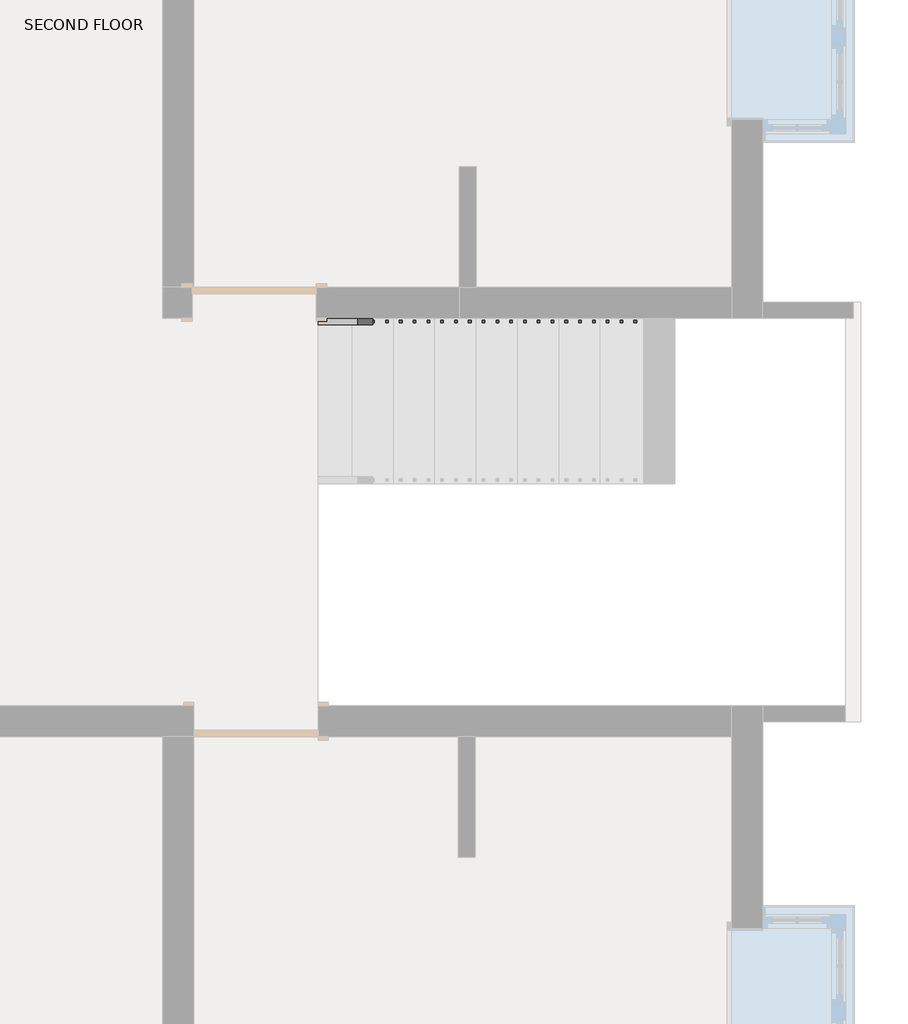
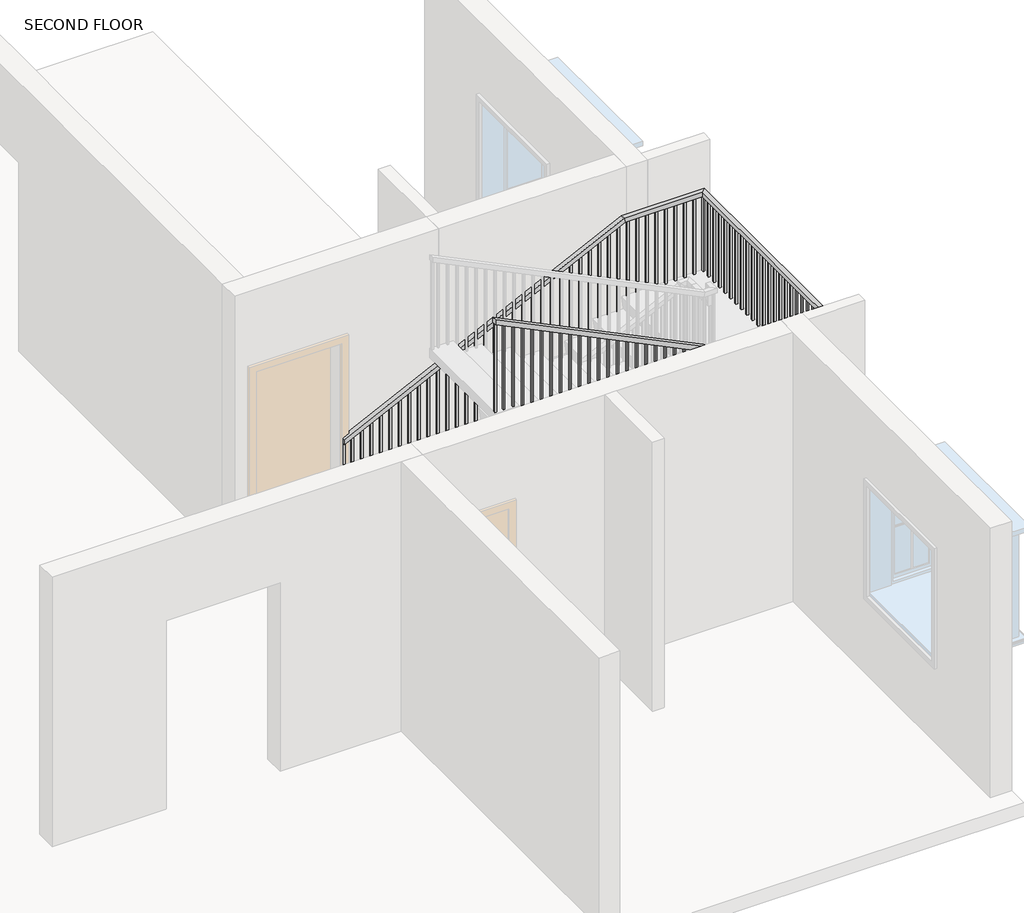
# One storey, part 4 of 6: 1 railing.
"""IFC4 building model written with IfcOpenShell, lengths in millimetres."""

from ifc_helpers import new_model, si_unit, frame, origin, place, context, project, spatial, polyline, outline, extrude, faceted_brep, element, save

model = new_model("IFC4")

# Units and contexts
model_context = context("Model", 3, world=origin())
ifc_project = project(units=[si_unit("LENGTHUNIT", "METRE", prefix="MILLI")], contexts=[model_context])

# Site, building, storey
site = spatial("IfcSite", under=ifc_project)
building = spatial("IfcBuilding", under=site)
storey = spatial("IfcBuildingStorey", under=building, Name="SECOND FLOOR", Elevation=6400.8)

# Railing
placement = place(None, origin())
element("IfcRailing", 1, ObjectType="Handrail - Rectangular", at=placement, inside=storey, context=model_context, shape_type="SolidModel", body=[
    faceted_brep([(3126.2584916, 220.733346, 7460.6727273), (3126.2584916, 220.733346, 7404.1956113), (3126.2584916, 169.933346, 7404.1956113), (3126.2584916, 169.933346, 7460.6727273), (6120.7829507, 220.733346, 8915.4), (6132.4691705, 220.733346, 8864.6), (6132.4691705, 169.933346, 8864.6), (6120.7829507, 169.933346, 8915.4), (7009.1350459, 220.733346, 8915.4), (7009.1350459, 220.733346, 8864.6), (6958.3350459, 169.933346, 8864.6), (6958.3350459, 169.933346, 8915.4), (7009.1350459, -2636.766654, 8915.4), (7009.1350459, -2636.766654, 8864.6), (6958.3350459, -2585.966654, 8864.6), (6958.3350459, -2585.966654, 8915.4), (6420.2353966, -2636.766654, 8915.4), (6408.5491768, -2636.766654, 8864.6), (6408.5491768, -2585.966654, 8864.6), (6420.2353966, -2585.966654, 8915.4), (3126.2584916, -2636.766654, 10515.6), (3126.2584916, -2585.966654, 10515.6), (3126.2584916, -2585.966654, 10459.122884), (3126.2584916, -2636.766654, 10459.122884)], [[[0, 1, 2, 3]], [[1, 0, 4, 5]], [[2, 1, 5, 6]], [[3, 2, 6, 7]], [[0, 3, 7, 4]], [[5, 4, 8, 9]], [[6, 5, 9, 10]], [[7, 6, 10, 11]], [[4, 7, 11, 8]], [[9, 8, 12, 13]], [[10, 9, 13, 14]], [[11, 10, 14, 15]], [[8, 11, 15, 12]], [[13, 12, 16, 17]], [[14, 13, 17, 18]], [[15, 14, 18, 19]], [[12, 15, 19, 16]], [[20, 21, 22, 23]], [[17, 16, 20, 23]], [[18, 17, 23, 22]], [[19, 18, 22, 21]], [[16, 19, 21, 20]]]),
    extrude(outline(polyline([(10416.0077556, 3215.0100459), (9455.7272727, 3215.0100459), (9455.7272727, 3234.0600459), (10406.7533465, 3234.0600459), (10416.0077556, 3215.0100459)])), frame((0.0, -2620.891654, 0.0), z_axis=(0.0, 1.0, 0.0), x_axis=(0.0, 0.0, 1.0)), (0.0, 0.0, 1.0), 19.05),
    extrude(outline(polyline([(10366.6509068, 3316.6100459), (9455.7272727, 3316.6100459), (9455.7272727, 3335.6600459), (10357.3964977, 3335.6600459), (10366.6509068, 3316.6100459)])), frame((0.0, -2620.891654, 0.0), z_axis=(0.0, 1.0, 0.0), x_axis=(0.0, 0.0, 1.0)), (0.0, 0.0, 1.0), 19.05),
    extrude(outline(polyline([(10317.294058, 3418.2100459), (9310.2545455, 3418.2100459), (9310.2545455, 3437.2600459), (10308.0396489, 3437.2600459), (10317.294058, 3418.2100459)])), frame((0.0, -2620.891654, 0.0), z_axis=(0.0, 1.0, 0.0), x_axis=(0.0, 0.0, 1.0)), (0.0, 0.0, 1.0), 19.05),
    extrude(outline(polyline([(10267.9372093, 3519.8100459), (9310.2545455, 3519.8100459), (9310.2545455, 3538.8600459), (10258.6828001, 3538.8600459), (10267.9372093, 3519.8100459)])), frame((0.0, -2620.891654, 0.0), z_axis=(0.0, 1.0, 0.0), x_axis=(0.0, 0.0, 1.0)), (0.0, 0.0, 1.0), 19.05),
    extrude(outline(polyline([(10218.5803605, 3621.4100459), (9310.2545455, 3621.4100459), (9310.2545455, 3640.4600459), (10209.3259513, 3640.4600459), (10218.5803605, 3621.4100459)])), frame((0.0, -2620.891654, 0.0), z_axis=(0.0, 1.0, 0.0), x_axis=(0.0, 0.0, 1.0)), (0.0, 0.0, 1.0), 19.05),
    extrude(outline(polyline([(10169.2235117, 3723.0100459), (9164.7818182, 3723.0100459), (9164.7818182, 3742.0600459), (10159.9691025, 3742.0600459), (10169.2235117, 3723.0100459)])), frame((0.0, -2620.891654, 0.0), z_axis=(0.0, 1.0, 0.0), x_axis=(0.0, 0.0, 1.0)), (0.0, 0.0, 1.0), 19.05),
    extrude(outline(polyline([(10119.8666629, 3824.6100459), (9164.7818182, 3824.6100459), (9164.7818182, 3843.6600459), (10110.6122538, 3843.6600459), (10119.8666629, 3824.6100459)])), frame((0.0, -2620.891654, 0.0), z_axis=(0.0, 1.0, 0.0), x_axis=(0.0, 0.0, 1.0)), (0.0, 0.0, 1.0), 19.05),
    extrude(outline(polyline([(10070.5098141, 3926.2100459), (9164.7818182, 3926.2100459), (9164.7818182, 3945.2600459), (10061.255405, 3945.2600459), (10070.5098141, 3926.2100459)])), frame((0.0, -2620.891654, 0.0), z_axis=(0.0, 1.0, 0.0), x_axis=(0.0, 0.0, 1.0)), (0.0, 0.0, 1.0), 19.05),
    extrude(outline(polyline([(10021.1529653, 4027.8100459), (9019.3090909, 4027.8100459), (9019.3090909, 4046.8600459), (10011.8985562, 4046.8600459), (10021.1529653, 4027.8100459)])), frame((0.0, -2620.891654, 0.0), z_axis=(0.0, 1.0, 0.0), x_axis=(0.0, 0.0, 1.0)), (0.0, 0.0, 1.0), 19.05),
    extrude(outline(polyline([(9971.7961165, 4129.4100459), (9019.3090909, 4129.4100459), (9019.3090909, 4148.4600459), (9962.5417074, 4148.4600459), (9971.7961165, 4129.4100459)])), frame((0.0, -2620.891654, 0.0), z_axis=(0.0, 1.0, 0.0), x_axis=(0.0, 0.0, 1.0)), (0.0, 0.0, 1.0), 19.05),
    extrude(outline(polyline([(9922.4392678, 4231.0100459), (9019.3090909, 4231.0100459), (9019.3090909, 4250.0600459), (9913.1848586, 4250.0600459), (9922.4392678, 4231.0100459)])), frame((0.0, -2620.891654, 0.0), z_axis=(0.0, 1.0, 0.0), x_axis=(0.0, 0.0, 1.0)), (0.0, 0.0, 1.0), 19.05),
    extrude(outline(polyline([(9873.082419, 4332.6100459), (8873.8363636, 4332.6100459), (8873.8363636, 4351.6600459), (9863.8280098, 4351.6600459), (9873.082419, 4332.6100459)])), frame((0.0, -2620.891654, 0.0), z_axis=(0.0, 1.0, 0.0), x_axis=(0.0, 0.0, 1.0)), (0.0, 0.0, 1.0), 19.05),
    extrude(outline(polyline([(9823.7255702, 4434.2100459), (8873.8363636, 4434.2100459), (8873.8363636, 4453.2600459), (9814.471161, 4453.2600459), (9823.7255702, 4434.2100459)])), frame((0.0, -2620.891654, 0.0), z_axis=(0.0, 1.0, 0.0), x_axis=(0.0, 0.0, 1.0)), (0.0, 0.0, 1.0), 19.05),
    extrude(outline(polyline([(9774.3687214, 4535.8100459), (8873.8363636, 4535.8100459), (8873.8363636, 4554.8600459), (9765.1143123, 4554.8600459), (9774.3687214, 4535.8100459)])), frame((0.0, -2620.891654, 0.0), z_axis=(0.0, 1.0, 0.0), x_axis=(0.0, 0.0, 1.0)), (0.0, 0.0, 1.0), 19.05),
    extrude(outline(polyline([(9725.0118726, 4637.4100459), (8728.3636364, 4637.4100459), (8728.3636364, 4656.4600459), (9715.7574635, 4656.4600459), (9725.0118726, 4637.4100459)])), frame((0.0, -2620.891654, 0.0), z_axis=(0.0, 1.0, 0.0), x_axis=(0.0, 0.0, 1.0)), (0.0, 0.0, 1.0), 19.05),
    extrude(outline(polyline([(9675.6550238, 4739.0100459), (8728.3636364, 4739.0100459), (8728.3636364, 4758.0600459), (9666.4006147, 4758.0600459), (9675.6550238, 4739.0100459)])), frame((0.0, -2620.891654, 0.0), z_axis=(0.0, 1.0, 0.0), x_axis=(0.0, 0.0, 1.0)), (0.0, 0.0, 1.0), 19.05),
    extrude(outline(polyline([(9626.2981751, 4840.6100459), (8728.3636364, 4840.6100459), (8728.3636364, 4859.6600459), (9617.0437659, 4859.6600459), (9626.2981751, 4840.6100459)])), frame((0.0, -2620.891654, 0.0), z_axis=(0.0, 1.0, 0.0), x_axis=(0.0, 0.0, 1.0)), (0.0, 0.0, 1.0), 19.05),
    extrude(outline(polyline([(9576.9413263, 4942.2100459), (8582.8909091, 4942.2100459), (8582.8909091, 4961.2600459), (9567.6869171, 4961.2600459), (9576.9413263, 4942.2100459)])), frame((0.0, -2620.891654, 0.0), z_axis=(0.0, 1.0, 0.0), x_axis=(0.0, 0.0, 1.0)), (0.0, 0.0, 1.0), 19.05),
    extrude(outline(polyline([(9527.5844775, 5043.8100459), (8582.8909091, 5043.8100459), (8582.8909091, 5062.8600459), (9518.3300683, 5062.8600459), (9527.5844775, 5043.8100459)])), frame((0.0, -2620.891654, 0.0), z_axis=(0.0, 1.0, 0.0), x_axis=(0.0, 0.0, 1.0)), (0.0, 0.0, 1.0), 19.05),
    extrude(outline(polyline([(9478.2276287, 5145.4100459), (8582.8909091, 5145.4100459), (8582.8909091, 5164.4600459), (9468.9732196, 5164.4600459), (9478.2276287, 5145.4100459)])), frame((0.0, -2620.891654, 0.0), z_axis=(0.0, 1.0, 0.0), x_axis=(0.0, 0.0, 1.0)), (0.0, 0.0, 1.0), 19.05),
    extrude(outline(polyline([(9428.8707799, 5247.0100459), (8437.4181818, 5247.0100459), (8437.4181818, 5266.0600459), (9419.6163708, 5266.0600459), (9428.8707799, 5247.0100459)])), frame((0.0, -2620.891654, 0.0), z_axis=(0.0, 1.0, 0.0), x_axis=(0.0, 0.0, 1.0)), (0.0, 0.0, 1.0), 19.05),
    extrude(outline(polyline([(9379.5139311, 5348.6100459), (8437.4181818, 5348.6100459), (8437.4181818, 5367.6600459), (9370.259522, 5367.6600459), (9379.5139311, 5348.6100459)])), frame((0.0, -2620.891654, 0.0), z_axis=(0.0, 1.0, 0.0), x_axis=(0.0, 0.0, 1.0)), (0.0, 0.0, 1.0), 19.05),
    extrude(outline(polyline([(9330.1570823, 5450.2100459), (8437.4181818, 5450.2100459), (8437.4181818, 5469.2600459), (9320.9026732, 5469.2600459), (9330.1570823, 5450.2100459)])), frame((0.0, -2620.891654, 0.0), z_axis=(0.0, 1.0, 0.0), x_axis=(0.0, 0.0, 1.0)), (0.0, 0.0, 1.0), 19.05),
    extrude(outline(polyline([(9280.8002336, 5551.8100459), (8291.9454545, 5551.8100459), (8291.9454545, 5570.8600459), (9271.5458244, 5570.8600459), (9280.8002336, 5551.8100459)])), frame((0.0, -2620.891654, 0.0), z_axis=(0.0, 1.0, 0.0), x_axis=(0.0, 0.0, 1.0)), (0.0, 0.0, 1.0), 19.05),
    extrude(outline(polyline([(9231.4433848, 5653.4100459), (8291.9454545, 5653.4100459), (8291.9454545, 5672.4600459), (9222.1889756, 5672.4600459), (9231.4433848, 5653.4100459)])), frame((0.0, -2620.891654, 0.0), z_axis=(0.0, 1.0, 0.0), x_axis=(0.0, 0.0, 1.0)), (0.0, 0.0, 1.0), 19.05),
    extrude(outline(polyline([(9182.086536, 5755.0100459), (8291.9454545, 5755.0100459), (8291.9454545, 5774.0600459), (9172.8321268, 5774.0600459), (9182.086536, 5755.0100459)])), frame((0.0, -2620.891654, 0.0), z_axis=(0.0, 1.0, 0.0), x_axis=(0.0, 0.0, 1.0)), (0.0, 0.0, 1.0), 19.05),
    extrude(outline(polyline([(9132.7296872, 5856.6100459), (8146.4727273, 5856.6100459), (8146.4727273, 5875.6600459), (9123.4752781, 5875.6600459), (9132.7296872, 5856.6100459)])), frame((0.0, -2620.891654, 0.0), z_axis=(0.0, 1.0, 0.0), x_axis=(0.0, 0.0, 1.0)), (0.0, 0.0, 1.0), 19.05),
    extrude(outline(polyline([(9083.3728384, 5958.2100459), (8146.4727273, 5958.2100459), (8146.4727273, 5977.2600459), (9074.1184293, 5977.2600459), (9083.3728384, 5958.2100459)])), frame((0.0, -2620.891654, 0.0), z_axis=(0.0, 1.0, 0.0), x_axis=(0.0, 0.0, 1.0)), (0.0, 0.0, 1.0), 19.05),
    extrude(outline(polyline([(9034.0159896, 6059.8100459), (8146.4727273, 6059.8100459), (8146.4727273, 6078.8600459), (9024.7615805, 6078.8600459), (9034.0159896, 6059.8100459)])), frame((0.0, -2620.891654, 0.0), z_axis=(0.0, 1.0, 0.0), x_axis=(0.0, 0.0, 1.0)), (0.0, 0.0, 1.0), 19.05),
    extrude(outline(polyline([(8984.6591409, 6161.4100459), (8001.0, 6161.4100459), (8001.0, 6180.4600459), (8975.4047317, 6180.4600459), (8984.6591409, 6161.4100459)])), frame((0.0, -2620.891654, 0.0), z_axis=(0.0, 1.0, 0.0), x_axis=(0.0, 0.0, 1.0)), (0.0, 0.0, 1.0), 19.05),
    extrude(outline(polyline([(8935.3022921, 6263.0100459), (8001.0, 6263.0100459), (8001.0, 6282.0600459), (8926.0478829, 6282.0600459), (8935.3022921, 6263.0100459)])), frame((0.0, -2620.891654, 0.0), z_axis=(0.0, 1.0, 0.0), x_axis=(0.0, 0.0, 1.0)), (0.0, 0.0, 1.0), 19.05),
    extrude(outline(polyline([(8885.9454433, 6364.6100459), (8001.0, 6364.6100459), (8001.0, 6383.6600459), (8876.6910341, 6383.6600459), (8885.9454433, 6364.6100459)])), frame((0.0, -2620.891654, 0.0), z_axis=(0.0, 1.0, 0.0), x_axis=(0.0, 0.0, 1.0)), (0.0, 0.0, 1.0), 19.05),
    extrude(outline(polyline([(6485.2600459, -2620.891654), (6466.2100459, -2620.891654), (6466.2100459, -2601.841654), (6485.2600459, -2601.841654), (6485.2600459, -2620.891654)])), frame((0.0, 0.0, 8001.0), z_axis=(0.0, 0.0, 1.0), x_axis=(1.0, 0.0, 0.0)), (0.0, 0.0, 1.0), 863.6),
    extrude(outline(polyline([(6586.8600459, -2620.891654), (6567.8100459, -2620.891654), (6567.8100459, -2601.841654), (6586.8600459, -2601.841654), (6586.8600459, -2620.891654)])), frame((0.0, 0.0, 8001.0), z_axis=(0.0, 0.0, 1.0), x_axis=(1.0, 0.0, 0.0)), (0.0, 0.0, 1.0), 863.6),
    extrude(outline(polyline([(6688.4600459, -2620.891654), (6669.4100459, -2620.891654), (6669.4100459, -2601.841654), (6688.4600459, -2601.841654), (6688.4600459, -2620.891654)])), frame((0.0, 0.0, 8001.0), z_axis=(0.0, 0.0, 1.0), x_axis=(1.0, 0.0, 0.0)), (0.0, 0.0, 1.0), 863.6),
    extrude(outline(polyline([(6790.0600459, -2620.891654), (6771.0100459, -2620.891654), (6771.0100459, -2601.841654), (6790.0600459, -2601.841654), (6790.0600459, -2620.891654)])), frame((0.0, 0.0, 8001.0), z_axis=(0.0, 0.0, 1.0), x_axis=(1.0, 0.0, 0.0)), (0.0, 0.0, 1.0), 863.6),
    extrude(outline(polyline([(6891.6600459, -2620.891654), (6872.6100459, -2620.891654), (6872.6100459, -2601.841654), (6891.6600459, -2601.841654), (6891.6600459, -2620.891654)])), frame((0.0, 0.0, 8001.0), z_axis=(0.0, 0.0, 1.0), x_axis=(1.0, 0.0, 0.0)), (0.0, 0.0, 1.0), 863.6),
    extrude(outline(polyline([(6993.2600459, -2538.341654), (6993.2600459, -2557.391654), (6974.2100459, -2557.391654), (6974.2100459, -2538.341654), (6993.2600459, -2538.341654)])), frame((0.0, 0.0, 8001.0), z_axis=(0.0, 0.0, 1.0), x_axis=(1.0, 0.0, 0.0)), (0.0, 0.0, 1.0), 863.6),
    extrude(outline(polyline([(6993.2600459, -2436.741654), (6993.2600459, -2455.791654), (6974.2100459, -2455.791654), (6974.2100459, -2436.741654), (6993.2600459, -2436.741654)])), frame((0.0, 0.0, 8001.0), z_axis=(0.0, 0.0, 1.0), x_axis=(1.0, 0.0, 0.0)), (0.0, 0.0, 1.0), 863.6),
    extrude(outline(polyline([(6993.2600459, -2335.141654), (6993.2600459, -2354.191654), (6974.2100459, -2354.191654), (6974.2100459, -2335.141654), (6993.2600459, -2335.141654)])), frame((0.0, 0.0, 8001.0), z_axis=(0.0, 0.0, 1.0), x_axis=(1.0, 0.0, 0.0)), (0.0, 0.0, 1.0), 863.6),
    extrude(outline(polyline([(6993.2600459, -2233.541654), (6993.2600459, -2252.591654), (6974.2100459, -2252.591654), (6974.2100459, -2233.541654), (6993.2600459, -2233.541654)])), frame((0.0, 0.0, 8001.0), z_axis=(0.0, 0.0, 1.0), x_axis=(1.0, 0.0, 0.0)), (0.0, 0.0, 1.0), 863.6),
    extrude(outline(polyline([(6993.2600459, -2131.941654), (6993.2600459, -2150.991654), (6974.2100459, -2150.991654), (6974.2100459, -2131.941654), (6993.2600459, -2131.941654)])), frame((0.0, 0.0, 8001.0), z_axis=(0.0, 0.0, 1.0), x_axis=(1.0, 0.0, 0.0)), (0.0, 0.0, 1.0), 863.6),
    extrude(outline(polyline([(6993.2600459, -2030.341654), (6993.2600459, -2049.391654), (6974.2100459, -2049.391654), (6974.2100459, -2030.341654), (6993.2600459, -2030.341654)])), frame((0.0, 0.0, 8001.0), z_axis=(0.0, 0.0, 1.0), x_axis=(1.0, 0.0, 0.0)), (0.0, 0.0, 1.0), 863.6),
    extrude(outline(polyline([(6993.2600459, -1928.741654), (6993.2600459, -1947.791654), (6974.2100459, -1947.791654), (6974.2100459, -1928.741654), (6993.2600459, -1928.741654)])), frame((0.0, 0.0, 8001.0), z_axis=(0.0, 0.0, 1.0), x_axis=(1.0, 0.0, 0.0)), (0.0, 0.0, 1.0), 863.6),
    extrude(outline(polyline([(6993.2600459, -1827.141654), (6993.2600459, -1846.191654), (6974.2100459, -1846.191654), (6974.2100459, -1827.141654), (6993.2600459, -1827.141654)])), frame((0.0, 0.0, 8001.0), z_axis=(0.0, 0.0, 1.0), x_axis=(1.0, 0.0, 0.0)), (0.0, 0.0, 1.0), 863.6),
    extrude(outline(polyline([(6993.2600459, -1725.541654), (6993.2600459, -1744.591654), (6974.2100459, -1744.591654), (6974.2100459, -1725.541654), (6993.2600459, -1725.541654)])), frame((0.0, 0.0, 8001.0), z_axis=(0.0, 0.0, 1.0), x_axis=(1.0, 0.0, 0.0)), (0.0, 0.0, 1.0), 863.6),
    extrude(outline(polyline([(6993.2600459, -1623.941654), (6993.2600459, -1642.991654), (6974.2100459, -1642.991654), (6974.2100459, -1623.941654), (6993.2600459, -1623.941654)])), frame((0.0, 0.0, 8001.0), z_axis=(0.0, 0.0, 1.0), x_axis=(1.0, 0.0, 0.0)), (0.0, 0.0, 1.0), 863.6),
    extrude(outline(polyline([(6993.2600459, -1522.341654), (6993.2600459, -1541.391654), (6974.2100459, -1541.391654), (6974.2100459, -1522.341654), (6993.2600459, -1522.341654)])), frame((0.0, 0.0, 8001.0), z_axis=(0.0, 0.0, 1.0), x_axis=(1.0, 0.0, 0.0)), (0.0, 0.0, 1.0), 863.6),
    extrude(outline(polyline([(6993.2600459, -1420.741654), (6993.2600459, -1439.791654), (6974.2100459, -1439.791654), (6974.2100459, -1420.741654), (6993.2600459, -1420.741654)])), frame((0.0, 0.0, 8001.0), z_axis=(0.0, 0.0, 1.0), x_axis=(1.0, 0.0, 0.0)), (0.0, 0.0, 1.0), 863.6),
    extrude(outline(polyline([(6993.2600459, -1319.141654), (6993.2600459, -1338.191654), (6974.2100459, -1338.191654), (6974.2100459, -1319.141654), (6993.2600459, -1319.141654)])), frame((0.0, 0.0, 8001.0), z_axis=(0.0, 0.0, 1.0), x_axis=(1.0, 0.0, 0.0)), (0.0, 0.0, 1.0), 863.6),
    extrude(outline(polyline([(6993.2600459, -1217.541654), (6993.2600459, -1236.591654), (6974.2100459, -1236.591654), (6974.2100459, -1217.541654), (6993.2600459, -1217.541654)])), frame((0.0, 0.0, 8001.0), z_axis=(0.0, 0.0, 1.0), x_axis=(1.0, 0.0, 0.0)), (0.0, 0.0, 1.0), 863.6),
    extrude(outline(polyline([(6993.2600459, -1115.941654), (6993.2600459, -1134.991654), (6974.2100459, -1134.991654), (6974.2100459, -1115.941654), (6993.2600459, -1115.941654)])), frame((0.0, 0.0, 8001.0), z_axis=(0.0, 0.0, 1.0), x_axis=(1.0, 0.0, 0.0)), (0.0, 0.0, 1.0), 863.6),
    extrude(outline(polyline([(6993.2600459, -1014.341654), (6993.2600459, -1033.391654), (6974.2100459, -1033.391654), (6974.2100459, -1014.341654), (6993.2600459, -1014.341654)])), frame((0.0, 0.0, 8001.0), z_axis=(0.0, 0.0, 1.0), x_axis=(1.0, 0.0, 0.0)), (0.0, 0.0, 1.0), 863.6),
    extrude(outline(polyline([(6993.2600459, -912.741654), (6993.2600459, -931.791654), (6974.2100459, -931.791654), (6974.2100459, -912.741654), (6993.2600459, -912.741654)])), frame((0.0, 0.0, 8001.0), z_axis=(0.0, 0.0, 1.0), x_axis=(1.0, 0.0, 0.0)), (0.0, 0.0, 1.0), 863.6),
    extrude(outline(polyline([(6993.2600459, -811.141654), (6993.2600459, -830.191654), (6974.2100459, -830.191654), (6974.2100459, -811.141654), (6993.2600459, -811.141654)])), frame((0.0, 0.0, 8001.0), z_axis=(0.0, 0.0, 1.0), x_axis=(1.0, 0.0, 0.0)), (0.0, 0.0, 1.0), 863.6),
    extrude(outline(polyline([(6993.2600459, -709.541654), (6993.2600459, -728.591654), (6974.2100459, -728.591654), (6974.2100459, -709.541654), (6993.2600459, -709.541654)])), frame((0.0, 0.0, 8001.0), z_axis=(0.0, 0.0, 1.0), x_axis=(1.0, 0.0, 0.0)), (0.0, 0.0, 1.0), 863.6),
    extrude(outline(polyline([(6993.2600459, -607.941654), (6993.2600459, -626.991654), (6974.2100459, -626.991654), (6974.2100459, -607.941654), (6993.2600459, -607.941654)])), frame((0.0, 0.0, 8001.0), z_axis=(0.0, 0.0, 1.0), x_axis=(1.0, 0.0, 0.0)), (0.0, 0.0, 1.0), 863.6),
    extrude(outline(polyline([(6993.2600459, -506.341654), (6993.2600459, -525.391654), (6974.2100459, -525.391654), (6974.2100459, -506.341654), (6993.2600459, -506.341654)])), frame((0.0, 0.0, 8001.0), z_axis=(0.0, 0.0, 1.0), x_axis=(1.0, 0.0, 0.0)), (0.0, 0.0, 1.0), 863.6),
    extrude(outline(polyline([(6993.2600459, -404.741654), (6993.2600459, -423.791654), (6974.2100459, -423.791654), (6974.2100459, -404.741654), (6993.2600459, -404.741654)])), frame((0.0, 0.0, 8001.0), z_axis=(0.0, 0.0, 1.0), x_axis=(1.0, 0.0, 0.0)), (0.0, 0.0, 1.0), 863.6),
    extrude(outline(polyline([(6993.2600459, -303.141654), (6993.2600459, -322.191654), (6974.2100459, -322.191654), (6974.2100459, -303.141654), (6993.2600459, -303.141654)])), frame((0.0, 0.0, 8001.0), z_axis=(0.0, 0.0, 1.0), x_axis=(1.0, 0.0, 0.0)), (0.0, 0.0, 1.0), 863.6),
    extrude(outline(polyline([(6993.2600459, -201.541654), (6993.2600459, -220.591654), (6974.2100459, -220.591654), (6974.2100459, -201.541654), (6993.2600459, -201.541654)])), frame((0.0, 0.0, 8001.0), z_axis=(0.0, 0.0, 1.0), x_axis=(1.0, 0.0, 0.0)), (0.0, 0.0, 1.0), 863.6),
    extrude(outline(polyline([(6993.2600459, -99.941654), (6993.2600459, -118.991654), (6974.2100459, -118.991654), (6974.2100459, -99.941654), (6993.2600459, -99.941654)])), frame((0.0, 0.0, 8001.0), z_axis=(0.0, 0.0, 1.0), x_axis=(1.0, 0.0, 0.0)), (0.0, 0.0, 1.0), 863.6),
    extrude(outline(polyline([(6993.2600459, 1.658346), (6993.2600459, -17.391654), (6974.2100459, -17.391654), (6974.2100459, 1.658346), (6993.2600459, 1.658346)])), frame((0.0, 0.0, 8001.0), z_axis=(0.0, 0.0, 1.0), x_axis=(1.0, 0.0, 0.0)), (0.0, 0.0, 1.0), 863.6),
    extrude(outline(polyline([(6993.2600459, 103.258346), (6993.2600459, 84.208346), (6974.2100459, 84.208346), (6974.2100459, 103.258346), (6993.2600459, 103.258346)])), frame((0.0, 0.0, 8001.0), z_axis=(0.0, 0.0, 1.0), x_axis=(1.0, 0.0, 0.0)), (0.0, 0.0, 1.0), 863.6),
    extrude(outline(polyline([(6875.9334916, 204.858346), (6894.9834916, 204.858346), (6894.9834916, 185.808346), (6875.9334916, 185.808346), (6875.9334916, 204.858346)])), frame((0.0, 0.0, 8001.0), z_axis=(0.0, 0.0, 1.0), x_axis=(1.0, 0.0, 0.0)), (0.0, 0.0, 1.0), 863.6),
    extrude(outline(polyline([(6774.3334916, 204.858346), (6793.3834916, 204.858346), (6793.3834916, 185.808346), (6774.3334916, 185.808346), (6774.3334916, 204.858346)])), frame((0.0, 0.0, 8001.0), z_axis=(0.0, 0.0, 1.0), x_axis=(1.0, 0.0, 0.0)), (0.0, 0.0, 1.0), 863.6),
    extrude(outline(polyline([(6672.7334916, 204.858346), (6691.7834916, 204.858346), (6691.7834916, 185.808346), (6672.7334916, 185.808346), (6672.7334916, 204.858346)])), frame((0.0, 0.0, 8001.0), z_axis=(0.0, 0.0, 1.0), x_axis=(1.0, 0.0, 0.0)), (0.0, 0.0, 1.0), 863.6),
    extrude(outline(polyline([(6571.1334916, 204.858346), (6590.1834916, 204.858346), (6590.1834916, 185.808346), (6571.1334916, 185.808346), (6571.1334916, 204.858346)])), frame((0.0, 0.0, 8001.0), z_axis=(0.0, 0.0, 1.0), x_axis=(1.0, 0.0, 0.0)), (0.0, 0.0, 1.0), 863.6),
    extrude(outline(polyline([(6469.5334916, 204.858346), (6488.5834916, 204.858346), (6488.5834916, 185.808346), (6469.5334916, 185.808346), (6469.5334916, 204.858346)])), frame((0.0, 0.0, 8001.0), z_axis=(0.0, 0.0, 1.0), x_axis=(1.0, 0.0, 0.0)), (0.0, 0.0, 1.0), 863.6),
    extrude(outline(polyline([(6367.9334916, 204.858346), (6386.9834916, 204.858346), (6386.9834916, 185.808346), (6367.9334916, 185.808346), (6367.9334916, 204.858346)])), frame((0.0, 0.0, 8001.0), z_axis=(0.0, 0.0, 1.0), x_axis=(1.0, 0.0, 0.0)), (0.0, 0.0, 1.0), 863.6),
    extrude(outline(polyline([(6266.3334916, 204.858346), (6285.3834916, 204.858346), (6285.3834916, 185.808346), (6266.3334916, 185.808346), (6266.3334916, 204.858346)])), frame((0.0, 0.0, 8001.0), z_axis=(0.0, 0.0, 1.0), x_axis=(1.0, 0.0, 0.0)), (0.0, 0.0, 1.0), 863.6),
    extrude(outline(polyline([(6164.7334916, 204.858346), (6183.7834916, 204.858346), (6183.7834916, 185.808346), (6164.7334916, 185.808346), (6164.7334916, 204.858346)])), frame((0.0, 0.0, 8001.0), z_axis=(0.0, 0.0, 1.0), x_axis=(1.0, 0.0, 0.0)), (0.0, 0.0, 1.0), 863.6),
    extrude(outline(polyline([(8830.9170215, 6063.1334916), (7855.5272727, 6063.1334916), (7855.5272727, 6082.1834916), (8840.1714306, 6082.1834916), (8830.9170215, 6063.1334916)])), frame((0.0, 185.808346, 0.0), z_axis=(0.0, 1.0, 0.0), x_axis=(0.0, 0.0, 1.0)), (0.0, 0.0, 1.0), 19.05),
    extrude(outline(polyline([(8781.5601727, 5961.5334916), (7855.5272727, 5961.5334916), (7855.5272727, 5980.5834916), (8790.8145818, 5980.5834916), (8781.5601727, 5961.5334916)])), frame((0.0, 185.808346, 0.0), z_axis=(0.0, 1.0, 0.0), x_axis=(0.0, 0.0, 1.0)), (0.0, 0.0, 1.0), 19.05),
    extrude(outline(polyline([(8732.2033239, 5859.9334916), (7855.5272727, 5859.9334916), (7855.5272727, 5878.9834916), (8741.457733, 5878.9834916), (8732.2033239, 5859.9334916)])), frame((0.0, 185.808346, 0.0), z_axis=(0.0, 1.0, 0.0), x_axis=(0.0, 0.0, 1.0)), (0.0, 0.0, 1.0), 19.05),
    extrude(outline(polyline([(8682.8464751, 5758.3334916), (7710.0545455, 5758.3334916), (7710.0545455, 5777.3834916), (8692.1008843, 5777.3834916), (8682.8464751, 5758.3334916)])), frame((0.0, 185.808346, 0.0), z_axis=(0.0, 1.0, 0.0), x_axis=(0.0, 0.0, 1.0)), (0.0, 0.0, 1.0), 19.05),
    extrude(outline(polyline([(8633.4896263, 5656.7334916), (7710.0545455, 5656.7334916), (7710.0545455, 5675.7834916), (8642.7440355, 5675.7834916), (8633.4896263, 5656.7334916)])), frame((0.0, 185.808346, 0.0), z_axis=(0.0, 1.0, 0.0), x_axis=(0.0, 0.0, 1.0)), (0.0, 0.0, 1.0), 19.05),
    extrude(outline(polyline([(8584.1327775, 5555.1334916), (7710.0545455, 5555.1334916), (7710.0545455, 5574.1834916), (8593.3871867, 5574.1834916), (8584.1327775, 5555.1334916)])), frame((0.0, 185.808346, 0.0), z_axis=(0.0, 1.0, 0.0), x_axis=(0.0, 0.0, 1.0)), (0.0, 0.0, 1.0), 19.05),
    extrude(outline(polyline([(8534.7759288, 5453.5334916), (7564.5818182, 5453.5334916), (7564.5818182, 5472.5834916), (8544.0303379, 5472.5834916), (8534.7759288, 5453.5334916)])), frame((0.0, 185.808346, 0.0), z_axis=(0.0, 1.0, 0.0), x_axis=(0.0, 0.0, 1.0)), (0.0, 0.0, 1.0), 19.05),
    extrude(outline(polyline([(8485.41908, 5351.9334916), (7564.5818182, 5351.9334916), (7564.5818182, 5370.9834916), (8494.6734891, 5370.9834916), (8485.41908, 5351.9334916)])), frame((0.0, 185.808346, 0.0), z_axis=(0.0, 1.0, 0.0), x_axis=(0.0, 0.0, 1.0)), (0.0, 0.0, 1.0), 19.05),
    extrude(outline(polyline([(8436.0622312, 5250.3334916), (7564.5818182, 5250.3334916), (7564.5818182, 5269.3834916), (8445.3166403, 5269.3834916), (8436.0622312, 5250.3334916)])), frame((0.0, 185.808346, 0.0), z_axis=(0.0, 1.0, 0.0), x_axis=(0.0, 0.0, 1.0)), (0.0, 0.0, 1.0), 19.05),
    extrude(outline(polyline([(8386.7053824, 5148.7334916), (7419.1090909, 5148.7334916), (7419.1090909, 5167.7834916), (8395.9597915, 5167.7834916), (8386.7053824, 5148.7334916)])), frame((0.0, 185.808346, 0.0), z_axis=(0.0, 1.0, 0.0), x_axis=(0.0, 0.0, 1.0)), (0.0, 0.0, 1.0), 19.05),
    extrude(outline(polyline([(8337.3485336, 5047.1334916), (7419.1090909, 5047.1334916), (7419.1090909, 5066.1834916), (8346.6029428, 5066.1834916), (8337.3485336, 5047.1334916)])), frame((0.0, 185.808346, 0.0), z_axis=(0.0, 1.0, 0.0), x_axis=(0.0, 0.0, 1.0)), (0.0, 0.0, 1.0), 19.05),
    extrude(outline(polyline([(8287.9916848, 4945.5334916), (7419.1090909, 4945.5334916), (7419.1090909, 4964.5834916), (8297.246094, 4964.5834916), (8287.9916848, 4945.5334916)])), frame((0.0, 185.808346, 0.0), z_axis=(0.0, 1.0, 0.0), x_axis=(0.0, 0.0, 1.0)), (0.0, 0.0, 1.0), 19.05),
    extrude(outline(polyline([(8238.634836, 4843.9334916), (7273.6363636, 4843.9334916), (7273.6363636, 4862.9834916), (8247.8892452, 4862.9834916), (8238.634836, 4843.9334916)])), frame((0.0, 185.808346, 0.0), z_axis=(0.0, 1.0, 0.0), x_axis=(0.0, 0.0, 1.0)), (0.0, 0.0, 1.0), 19.05),
    extrude(outline(polyline([(8189.2779873, 4742.3334916), (7273.6363636, 4742.3334916), (7273.6363636, 4761.3834916), (8198.5323964, 4761.3834916), (8189.2779873, 4742.3334916)])), frame((0.0, 185.808346, 0.0), z_axis=(0.0, 1.0, 0.0), x_axis=(0.0, 0.0, 1.0)), (0.0, 0.0, 1.0), 19.05),
    extrude(outline(polyline([(8139.9211385, 4640.7334916), (7273.6363636, 4640.7334916), (7273.6363636, 4659.7834916), (8149.1755476, 4659.7834916), (8139.9211385, 4640.7334916)])), frame((0.0, 185.808346, 0.0), z_axis=(0.0, 1.0, 0.0), x_axis=(0.0, 0.0, 1.0)), (0.0, 0.0, 1.0), 19.05),
    extrude(outline(polyline([(8090.5642897, 4539.1334916), (7128.1636364, 4539.1334916), (7128.1636364, 4558.1834916), (8099.8186988, 4558.1834916), (8090.5642897, 4539.1334916)])), frame((0.0, 185.808346, 0.0), z_axis=(0.0, 1.0, 0.0), x_axis=(0.0, 0.0, 1.0)), (0.0, 0.0, 1.0), 19.05),
    extrude(outline(polyline([(8041.2074409, 4437.5334916), (7128.1636364, 4437.5334916), (7128.1636364, 4456.5834916), (8050.4618501, 4456.5834916), (8041.2074409, 4437.5334916)])), frame((0.0, 185.808346, 0.0), z_axis=(0.0, 1.0, 0.0), x_axis=(0.0, 0.0, 1.0)), (0.0, 0.0, 1.0), 19.05),
    extrude(outline(polyline([(7991.8505921, 4335.9334916), (7128.1636364, 4335.9334916), (7128.1636364, 4354.9834916), (8001.1050013, 4354.9834916), (7991.8505921, 4335.9334916)])), frame((0.0, 185.808346, 0.0), z_axis=(0.0, 1.0, 0.0), x_axis=(0.0, 0.0, 1.0)), (0.0, 0.0, 1.0), 19.05),
    extrude(outline(polyline([(7942.4937433, 4234.3334916), (6982.6909091, 4234.3334916), (6982.6909091, 4253.3834916), (7951.7481525, 4253.3834916), (7942.4937433, 4234.3334916)])), frame((0.0, 185.808346, 0.0), z_axis=(0.0, 1.0, 0.0), x_axis=(0.0, 0.0, 1.0)), (0.0, 0.0, 1.0), 19.05),
    extrude(outline(polyline([(7893.1368946, 4132.7334916), (6982.6909091, 4132.7334916), (6982.6909091, 4151.7834916), (7902.3913037, 4151.7834916), (7893.1368946, 4132.7334916)])), frame((0.0, 185.808346, 0.0), z_axis=(0.0, 1.0, 0.0), x_axis=(0.0, 0.0, 1.0)), (0.0, 0.0, 1.0), 19.05),
    extrude(outline(polyline([(7843.7800458, 4031.1334916), (6982.6909091, 4031.1334916), (6982.6909091, 4050.1834916), (7853.0344549, 4050.1834916), (7843.7800458, 4031.1334916)])), frame((0.0, 185.808346, 0.0), z_axis=(0.0, 1.0, 0.0), x_axis=(0.0, 0.0, 1.0)), (0.0, 0.0, 1.0), 19.05),
    extrude(outline(polyline([(7794.423197, 3929.5334916), (6837.2181818, 3929.5334916), (6837.2181818, 3948.5834916), (7803.6776061, 3948.5834916), (7794.423197, 3929.5334916)])), frame((0.0, 185.808346, 0.0), z_axis=(0.0, 1.0, 0.0), x_axis=(0.0, 0.0, 1.0)), (0.0, 0.0, 1.0), 19.05),
    extrude(outline(polyline([(7745.0663482, 3827.9334916), (6837.2181818, 3827.9334916), (6837.2181818, 3846.9834916), (7754.3207573, 3846.9834916), (7745.0663482, 3827.9334916)])), frame((0.0, 185.808346, 0.0), z_axis=(0.0, 1.0, 0.0), x_axis=(0.0, 0.0, 1.0)), (0.0, 0.0, 1.0), 19.05),
    extrude(outline(polyline([(7695.7094994, 3726.3334916), (6837.2181818, 3726.3334916), (6837.2181818, 3745.3834916), (7704.9639086, 3745.3834916), (7695.7094994, 3726.3334916)])), frame((0.0, 185.808346, 0.0), z_axis=(0.0, 1.0, 0.0), x_axis=(0.0, 0.0, 1.0)), (0.0, 0.0, 1.0), 19.05),
    extrude(outline(polyline([(7646.3526506, 3624.7334916), (6691.7454545, 3624.7334916), (6691.7454545, 3643.7834916), (7655.6070598, 3643.7834916), (7646.3526506, 3624.7334916)])), frame((0.0, 185.808346, 0.0), z_axis=(0.0, 1.0, 0.0), x_axis=(0.0, 0.0, 1.0)), (0.0, 0.0, 1.0), 19.05),
    extrude(outline(polyline([(7596.9958018, 3523.1334916), (6691.7454545, 3523.1334916), (6691.7454545, 3542.1834916), (7606.250211, 3542.1834916), (7596.9958018, 3523.1334916)])), frame((0.0, 185.808346, 0.0), z_axis=(0.0, 1.0, 0.0), x_axis=(0.0, 0.0, 1.0)), (0.0, 0.0, 1.0), 19.05),
    extrude(outline(polyline([(7547.6389531, 3421.5334916), (6691.7454545, 3421.5334916), (6691.7454545, 3440.5834916), (7556.8933622, 3440.5834916), (7547.6389531, 3421.5334916)])), frame((0.0, 185.808346, 0.0), z_axis=(0.0, 1.0, 0.0), x_axis=(0.0, 0.0, 1.0)), (0.0, 0.0, 1.0), 19.05),
    extrude(outline(polyline([(7498.2821043, 3319.9334916), (6546.2727273, 3319.9334916), (6546.2727273, 3338.9834916), (7507.5365134, 3338.9834916), (7498.2821043, 3319.9334916)])), frame((0.0, 185.808346, 0.0), z_axis=(0.0, 1.0, 0.0), x_axis=(0.0, 0.0, 1.0)), (0.0, 0.0, 1.0), 19.05),
    extrude(outline(polyline([(7448.9252555, 3218.3334916), (6546.2727273, 3218.3334916), (6546.2727273, 3237.3834916), (7458.1796646, 3237.3834916), (7448.9252555, 3218.3334916)])), frame((0.0, 185.808346, 0.0), z_axis=(0.0, 1.0, 0.0), x_axis=(0.0, 0.0, 1.0)), (0.0, 0.0, 1.0), 19.05),
    extrude(outline(polyline([(6993.2600459, -2601.841654), (6993.2600459, -2620.891654), (6974.2100459, -2620.891654), (6974.2100459, -2601.841654), (6993.2600459, -2601.841654)])), frame((0.0, 0.0, 8001.0), z_axis=(0.0, 0.0, 1.0), x_axis=(1.0, 0.0, 0.0)), (0.0, 0.0, 1.0), 863.6),
    extrude(outline(polyline([(6974.2100459, 204.858346), (6993.2600459, 204.858346), (6993.2600459, 185.808346), (6974.2100459, 185.808346), (6974.2100459, 204.858346)])), frame((0.0, 0.0, 8001.0), z_axis=(0.0, 0.0, 1.0), x_axis=(1.0, 0.0, 0.0)), (0.0, 0.0, 1.0), 863.6),
    extrude(outline(polyline([(10459.122884, 3126.2584916), (9455.7272727, 3126.2584916), (9455.7272727, 3145.3084916), (10449.8684749, 3145.3084916), (10459.122884, 3126.2584916)])), frame((0.0, -2620.891654, 0.0), z_axis=(0.0, 1.0, 0.0), x_axis=(0.0, 0.0, 1.0)), (0.0, 0.0, 1.0), 19.05),
    extrude(outline(polyline([(7404.1956113, 3126.2584916), (6546.2727273, 3126.2584916), (6546.2727273, 3145.3084916), (7413.4500204, 3145.3084916), (7404.1956113, 3126.2584916)])), frame((0.0, 185.808346, 0.0), z_axis=(0.0, 1.0, 0.0), x_axis=(0.0, 0.0, 1.0)), (0.0, 0.0, 1.0), 19.05),
])

save(model, "model.ifc")

# Revit data of these elements
# Type "Handrail - Rectangular"
#   Assembly Code = "C2010400"
#   built-in parameter 1008612 = 0.0416667 (stored number, unit not read)
#   built-in parameter 1008611 = 0.0416667 (stored number, unit not read)
#   built-in parameter 1008609 = 0.333333 (stored number, unit not read)
#   built-in parameter 1008604 = 0.166667 (stored number, unit not read)
#   built-in parameter 1008603 = 0.166667 (stored number, unit not read)
#   Railing Height = 3' - 0"
#   built-in parameter 1008630 = 2
#   built-in parameter 1008610 = 2
#   built-in parameter 1008618 = Baluster - Square : 3/4"
# Element 1 (IfcRailing, "Handrail - Rectangular")
#   Phase Created = New Construction
